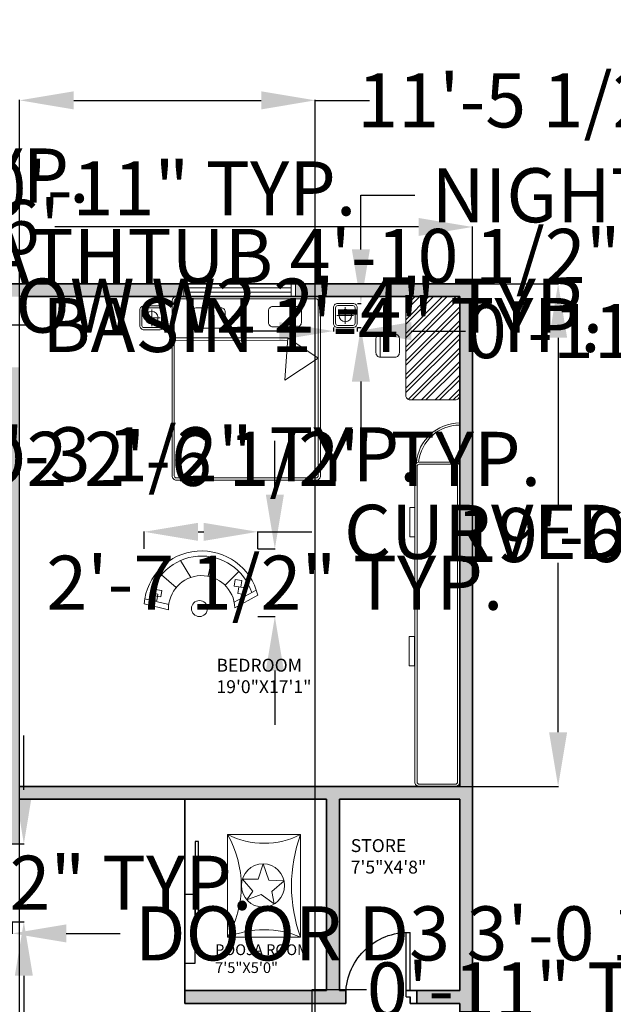
# Model space of a CAD drawing. Units: inches. Extents: x 35 to 5908, y 4 to 3165.
# Tile 5 of 6: x 5270 to 5546, y 2706 to 3165. Entities that reach past the tile are written whole.
import ezdxf

# ---------------------------------------------------------------- set-up
doc = ezdxf.new("R2010")
doc.units = ezdxf.units.IN
doc.header["$MEASUREMENT"] = 0
for name, color, linetype, lineweight in [('A-ANNO-DIMS', 2, 'Continuous', 18), ('A-DOOR', 4, 'Continuous', 25), ('A-FLOR-CASE', 8, 'Continuous', 18), ('A-FURN', 8, 'Continuous', 18), ('A-FURN-PATT', 9, 'Continuous', 13), ('A-WALL', 7, 'Continuous', 35), ('A-WALL-PATT', 252, 'Continuous', 13)]:
    doc.layers.add(name, color=color, linetype=linetype, lineweight=lineweight)
doc.layers.add('A-AREA-IDEN', color=30, linetype='Continuous', lineweight=18, true_color=0xf8991e)
doc.layers.add('A-GLAZ', color=30, linetype='Continuous', lineweight=18, true_color=0xf8991e)
doc.styles.get("Standard").update_dxf_attribs({"font": 'arial.ttf'})
doc.dimstyles.get("Standard").update_dxf_attribs({"dimtxt": 25.18, "dimasz": 25.18, "dimexe": 0.18, "dimexo": 0.0625, "dimgap": 0.09, "dimtad": 0, "dimtih": 1, "dimtoh": 1, "dimdec": 0, "dimzin": 0, "dimdsep": 46, "dimlunit": 3, "dimtxsty": 'Standard', "dimcen": 0.09, "dimadec": 0, "dimazin": 0, "dimtfac": 1, "dimtdec": 0, "dimtofl": 0, "dimtmove": 0, "dimatfit": 3, "dimfxl": 1, "dimtolj": 1, "dimtzin": 0, "dimarcsym": 0})

# ---------------------------------------------------------------- blocks, each defined once
blk = doc.blocks.new('*D6')
at = {"layer": 'A-ANNO-DIMS', "color": 0, "lineweight": -2, "transparency": 16777216}
for p, q in [((5048.79, 3041.84), (5048.79, 3068.36)), ((5073.97, 3068.18), (5243.35, 3068.18)), ((5455.61, 3068.18), (5286.24, 3068.18)), ((5480.79, 3041.84), (5480.79, 3068.36))]:
    blk.add_line(p, q, dxfattribs=at)
for points in [[(5073.97, 3072.38), (5073.97, 3063.99), (5048.79, 3068.18)], [(5455.61, 3072.38), (5455.61, 3063.99), (5480.79, 3068.18)]]:
    blk.add_solid(points, dxfattribs=at)
at = {"layer": 'Defpoints', "color": 0, "lineweight": -2, "transparency": 16777216}
for p in [(5480.79, 3068.18), (5048.79, 3041.78), (5480.79, 3041.78)]:
    blk.add_point(p, dxfattribs=at)
at = {"layer": 'A-ANNO-DIMS', "color": 0, "transparency": 16777216, "insert": (5264.79, 3068.18), "char_height": 25.18, "attachment_point": 5}
blk.add_mtext("\\A1;36'", dxfattribs=at)
blk = doc.blocks.new('DOOR-30-3-JAMB')
for p, q in [((-2, -27), (-2, 0)), ((0, -30), (0, 0)), ((0, -30), (-2, -30))]:
    blk.add_line(p, q)
blk.add_arc((-1, -29), 29.02, 358.0251, 91.9749)
blk = doc.blocks.new('WINDOW-48')
for p, q in [((0, 0), (0, 6)), ((2, 0), (2, 6)), ((50, 0), (50, 6)), ((52, 0), (52, 6)), ((2, 4), (50, 4)), ((2, 2), (50, 2))]:
    blk.add_line(p, q)
blk = doc.blocks.new('NIGHTSTAND-SQUARE')
for p, q in [((-3.9, 0), (3.83, 0)), ((-0.03, 3.86), (-0.03, -3.96))]:
    blk.add_line(p, q)
for points in [[(-5.56, 3.6, -0.414214), (-3.56, 5.6), (3.56, 5.6, -0.414214), (5.56, 3.6), (5.56, -3.6, -0.414214), (3.56, -5.6), (-3.56, -5.6, -0.414214), (-5.56, -3.6)], [(-4.56, 3.6, -0.414214), (-3.56, 4.6), (3.56, 4.6, -0.414214), (4.56, 3.6), (4.56, -3.6, -0.414214), (3.56, -4.6), (-3.56, -4.6, -0.414214), (-4.56, -3.6)]]:
    blk.add_lwpolyline(points, format="xyb", close=True)
blk.add_circle((0, 0), 2.93)
blk = doc.blocks.new('SEATING-SEMICIRCULAR')
for p, q in [((-8.61, 26.49), (-2.9, 16.18)), ((-6.26, 27.18), (-0.33, 16.47)), ((-10.8, 11.96), (-17.22, 18.38)), ((-15.03, 4.08), (-23.93, 5.87)), ((-14.47, -4.08), (-22.37, -8.78)), ((-9.84, -10.8), (-15.69, -17.74)), ((-4.52, -25.5), (-1.86, -14.3)), ((-2.14, -25.8), (0.56, -14.43))]:
    blk.add_line(p, q)
for points in [[(-12.99, 19.72), (-13.45, 16.67), (-10.4, 16.21), (-9.94, 19.26)], [(-9.61, 21.43), (-10.07, 18.38), (-7.03, 17.91), (-6.56, 20.96)], [(-8.44, -17.54), (-8.91, -20.58), (-5.86, -21.05), (-5.4, -18)], [(-6.7, -19.36), (-7.17, -22.4), (-4.12, -22.87), (-3.66, -19.82)]]:
    blk.add_lwpolyline(points, close=True)
blk.add_circle((0, 0), 3.73)
for radius, start, end in [(26.92, 103.6927, 265.1976), (24.53, 107.9155, 260.4199), (15.45, 91.6667, 271.6667)]:
    blk.add_arc((0.12, 1.02), radius, start, end)
blk = doc.blocks.new('*D20')
at = {"layer": 'A-ANNO-DIMS', "color": 0, "lineweight": -2, "transparency": 16777216}
for p, q in [((5366.93, 2650.28), (5341.75, 2650.28)), ((5392.11, 2652.05), (5392.11, 2650.1)), ((5404.3, 2652.05), (5404.3, 2650.1)), ((5429.48, 2650.28), (5454.66, 2650.28))]:
    blk.add_line(p, q, dxfattribs=at)
for points in [[(5366.93, 2654.48), (5366.93, 2646.08), (5392.11, 2650.28)], [(5429.48, 2654.48), (5429.48, 2646.08), (5404.3, 2650.28)]]:
    blk.add_solid(points, dxfattribs=at)
at = {"layer": 'Defpoints', "color": 0, "lineweight": -2, "transparency": 16777216}
for p in [(5392.11, 2652.11), (5404.3, 2652.11), (5404.3, 2650.28)]:
    blk.add_point(p, dxfattribs=at)
at = {"layer": 'A-ANNO-DIMS', "color": 0, "transparency": 16777216, "insert": (5656.92, 2650.28), "char_height": 25.18, "attachment_point": 5}
blk.add_mtext('\\A1;DINING CHAIR 1\'-0" TYP.', dxfattribs=at)
blk = doc.blocks.new('*D21')
at = {"layer": 'A-ANNO-DIMS', "color": 0, "lineweight": -2, "transparency": 16777216}
for p, q in [((5406.13, 2688.06), (5406.13, 2713.24)), ((5406.13, 2713.24), (5431.31, 2713.24)), ((5404.36, 2662.88), (5406.31, 2662.88)), ((5404.36, 2652.11), (5406.31, 2652.11)), ((5406.13, 2626.93), (5406.13, 2601.75))]:
    blk.add_line(p, q, dxfattribs=at)
for points in [[(5401.93, 2688.06), (5410.32, 2688.06), (5406.13, 2662.88)], [(5401.93, 2626.93), (5410.32, 2626.93), (5406.13, 2652.11)]]:
    blk.add_solid(points, dxfattribs=at)
at = {"layer": 'Defpoints', "color": 0, "lineweight": -2, "transparency": 16777216}
for p in [(5404.3, 2662.88), (5406.13, 2662.88), (5404.3, 2652.11)]:
    blk.add_point(p, dxfattribs=at)
at = {"layer": 'A-ANNO-DIMS', "color": 0, "transparency": 16777216, "insert": (5517.92, 2713.24), "char_height": 25.18, "attachment_point": 5}
blk.add_mtext('\\A1;0\'-11" TYP.', dxfattribs=at)
blk = doc.blocks.new('*D24')
at = {"layer": 'A-ANNO-DIMS', "color": 0, "lineweight": -2, "transparency": 16777216}
for p, q in [((5184.7, 3022.57), (5159.52, 3022.57)), ((5209.88, 3024.93), (5209.88, 3022.39)), ((5226.05, 3024.93), (5226.05, 3022.39)), ((5251.23, 3022.57), (5276.41, 3022.57))]:
    blk.add_line(p, q, dxfattribs=at)
for points in [[(5184.7, 3026.76), (5184.7, 3018.37), (5209.88, 3022.57)], [(5251.23, 3026.76), (5251.23, 3018.37), (5226.05, 3022.57)]]:
    blk.add_solid(points, dxfattribs=at)
at = {"layer": 'Defpoints', "color": 0, "lineweight": -2, "transparency": 16777216}
for p in [(5209.88, 3024.99), (5226.05, 3024.99), (5226.05, 3022.57)]:
    blk.add_point(p, dxfattribs=at)
at = {"layer": 'A-ANNO-DIMS', "color": 0, "transparency": 16777216, "insert": (5410.36, 3022.57), "char_height": 25.18, "attachment_point": 5}
blk.add_mtext('\\A1;BASIN 1\'-4" TYP.', dxfattribs=at)
blk = doc.blocks.new('*D25')
at = {"layer": 'A-ANNO-DIMS', "color": 0, "lineweight": -2, "transparency": 16777216}
for p, q in [((5228.48, 3060.96), (5228.48, 3086.14)), ((5228.48, 3086.14), (5253.66, 3086.14)), ((5226.12, 3035.78), (5228.66, 3035.78)), ((5226.12, 3024.99), (5228.66, 3024.99)), ((5228.48, 2999.81), (5228.48, 2974.63))]:
    blk.add_line(p, q, dxfattribs=at)
for points in [[(5224.28, 3060.96), (5232.68, 3060.96), (5228.48, 3035.78)], [(5224.28, 2999.81), (5232.68, 2999.81), (5228.48, 3024.99)]]:
    blk.add_solid(points, dxfattribs=at)
at = {"layer": 'Defpoints', "color": 0, "lineweight": -2, "transparency": 16777216}
for p in [(5226.05, 3035.78), (5228.48, 3035.78), (5226.05, 3024.99)]:
    blk.add_point(p, dxfattribs=at)
at = {"layer": 'A-ANNO-DIMS', "color": 0, "transparency": 16777216, "insert": (5340.27, 3086.14), "char_height": 25.18, "attachment_point": 5}
blk.add_mtext('\\A1;0\'-11" TYP.', dxfattribs=at)
blk = doc.blocks.new('*D28')
at = {"layer": 'A-ANNO-DIMS', "color": 0, "lineweight": -2, "transparency": 16777216}
for p, q in [((5091.29, 3035.72), (5091.29, 3031.4)), ((5119.29, 3035.72), (5119.29, 3031.4)), ((5066.11, 3031.58), (5040.93, 3031.58)), ((5144.47, 3031.58), (5169.65, 3031.58))]:
    blk.add_line(p, q, dxfattribs=at)
for points in [[(5066.11, 3035.78), (5066.11, 3027.38), (5091.29, 3031.58)], [(5144.47, 3035.78), (5144.47, 3027.38), (5119.29, 3031.58)]]:
    blk.add_solid(points, dxfattribs=at)
at = {"layer": 'Defpoints', "color": 0, "lineweight": -2, "transparency": 16777216}
for p in [(5091.29, 3035.78), (5119.29, 3035.78), (5119.29, 3031.58)]:
    blk.add_point(p, dxfattribs=at)
at = {"layer": 'A-ANNO-DIMS', "color": 0, "transparency": 16777216, "insert": (5360.33, 3031.58), "char_height": 25.18, "attachment_point": 5}
blk.add_mtext('\\A1;WINDOW W2 2\'-4" TYP.', dxfattribs=at)
blk = doc.blocks.new('*D29')
at = {"layer": 'A-ANNO-DIMS', "color": 0, "lineweight": -2, "transparency": 16777216}
for p, q in [((5123.49, 3066.96), (5123.49, 3092.14)), ((5123.49, 3092.14), (5148.67, 3092.14)), ((5119.36, 3041.78), (5123.67, 3041.78)), ((5119.36, 3035.78), (5123.67, 3035.78)), ((5123.49, 3010.6), (5123.49, 2985.42))]:
    blk.add_line(p, q, dxfattribs=at)
for points in [[(5119.3, 3066.96), (5127.69, 3066.96), (5123.49, 3041.78)], [(5119.3, 3010.6), (5127.69, 3010.6), (5123.49, 3035.78)]]:
    blk.add_solid(points, dxfattribs=at)
at = {"layer": 'Defpoints', "color": 0, "lineweight": -2, "transparency": 16777216}
for p in [(5119.29, 3041.78), (5123.49, 3041.78), (5119.29, 3035.78)]:
    blk.add_point(p, dxfattribs=at)
at = {"layer": 'A-ANNO-DIMS', "color": 0, "transparency": 16777216, "insert": (5225.51, 3092.14), "char_height": 25.18, "attachment_point": 5}
blk.add_mtext('\\A1;0\'-6" TYP.', dxfattribs=at)
blk = doc.blocks.new('*D30')
at = {"layer": 'A-ANNO-DIMS', "color": 0, "lineweight": -2, "transparency": 16777216}
for p, q in [((5057.79, 2964.72), (5057.79, 2960.06)), ((5088.07, 2964.72), (5088.07, 2960.06)), ((5032.61, 2960.24), (5007.43, 2960.24)), ((5113.25, 2960.24), (5138.43, 2960.24))]:
    blk.add_line(p, q, dxfattribs=at)
for points in [[(5032.61, 2964.43), (5032.61, 2956.04), (5057.79, 2960.24)], [(5113.25, 2964.43), (5113.25, 2956.04), (5088.07, 2960.24)]]:
    blk.add_solid(points, dxfattribs=at)
at = {"layer": 'Defpoints', "color": 0, "lineweight": -2, "transparency": 16777216}
for p in [(5057.79, 2964.78), (5088.07, 2964.78), (5088.07, 2960.24)]:
    blk.add_point(p, dxfattribs=at)
at = {"layer": 'A-ANNO-DIMS', "color": 0, "transparency": 16777216, "insert": (5329, 2960.24), "char_height": 25.18, "attachment_point": 5}
blk.add_mtext('\\A1;DOOR D2 2\'-6 1/2" TYP.', dxfattribs=at)
blk = doc.blocks.new('*D32')
at = {"layer": 'A-ANNO-DIMS', "color": 0, "lineweight": -2, "transparency": 16777216}
for p, q in [((5230.02, 2744.72), (5230.02, 2739.16)), ((5266.29, 2744.72), (5266.29, 2739.16)), ((5204.84, 2739.34), (5179.66, 2739.34)), ((5291.47, 2739.34), (5316.65, 2739.34))]:
    blk.add_line(p, q, dxfattribs=at)
for points in [[(5204.84, 2743.53), (5204.84, 2735.14), (5230.02, 2739.34)], [(5291.47, 2743.53), (5291.47, 2735.14), (5266.29, 2739.34)]]:
    blk.add_solid(points, dxfattribs=at)
at = {"layer": 'Defpoints', "color": 0, "lineweight": -2, "transparency": 16777216}
for p in [(5230.02, 2744.78), (5266.29, 2744.78), (5266.29, 2739.34)]:
    blk.add_point(p, dxfattribs=at)
at = {"layer": 'A-ANNO-DIMS', "color": 0, "transparency": 16777216, "insert": (5507.22, 2739.34), "char_height": 25.18, "attachment_point": 5}
blk.add_mtext('\\A1;DOOR D3 3\'-0 1/2" TYP.', dxfattribs=at)
blk = doc.blocks.new('*D33')
at = {"layer": 'A-ANNO-DIMS', "color": 0, "lineweight": -2, "transparency": 16777216}
for p, q in [((5271.74, 2806.23), (5271.74, 2831.41)), ((5266.36, 2781.05), (5271.92, 2781.05)), ((5266.36, 2744.78), (5271.92, 2744.78)), ((5271.74, 2719.6), (5271.74, 2694.42))]:
    blk.add_line(p, q, dxfattribs=at)
for points in [[(5267.54, 2806.23), (5275.93, 2806.23), (5271.74, 2781.05)], [(5267.54, 2719.6), (5275.93, 2719.6), (5271.74, 2744.78)]]:
    blk.add_solid(points, dxfattribs=at)
at = {"layer": 'Defpoints', "color": 0, "lineweight": -2, "transparency": 16777216}
for p in [(5266.29, 2781.05), (5271.74, 2781.05), (5266.29, 2744.78)]:
    blk.add_point(p, dxfattribs=at)
at = {"layer": 'A-ANNO-DIMS', "color": 0, "transparency": 16777216, "insert": (5271.74, 2762.92), "char_height": 25.18, "attachment_point": 5}
blk.add_mtext('\\A1;3\'-0 1/2" TYP.', dxfattribs=at)
blk = doc.blocks.new('*D34')
at = {"layer": 'A-ANNO-DIMS', "color": 0, "lineweight": -2, "transparency": 16777216}
for p, q in [((5201.71, 3029.52), (5201.71, 3054.7)), ((5201.71, 3054.7), (5226.89, 3054.7)), ((5193.01, 3029.52), (5201.89, 3029.52)), ((5201.71, 2996.29), (5201.71, 3004.34)), ((5193.01, 2971.11), (5201.89, 2971.11))]:
    blk.add_line(p, q, dxfattribs=at)
for points in [[(5197.51, 3004.34), (5205.9, 3004.34), (5201.71, 3029.52)], [(5197.51, 2996.29), (5205.9, 2996.29), (5201.71, 2971.11)]]:
    blk.add_solid(points, dxfattribs=at)
at = {"layer": 'Defpoints', "color": 0, "lineweight": -2, "transparency": 16777216}
for p in [(5192.94, 3029.52), (5201.71, 3029.52), (5192.94, 2971.11)]:
    blk.add_point(p, dxfattribs=at)
at = {"layer": 'A-ANNO-DIMS', "color": 0, "transparency": 16777216, "insert": (5429.25, 3054.7), "char_height": 25.18, "attachment_point": 5}
blk.add_mtext('\\A1;BATHTUB 4\'-10 1/2" TYP.', dxfattribs=at)
blk = doc.blocks.new('*D35')
at = {"layer": 'A-ANNO-DIMS', "color": 0, "lineweight": -2, "transparency": 16777216}
for p, q in [((5165.59, 2971.05), (5165.59, 2962.17)), ((5192.94, 2971.05), (5192.94, 2962.17)), ((5140.41, 2962.35), (5115.23, 2962.35)), ((5218.12, 2962.35), (5243.3, 2962.35))]:
    blk.add_line(p, q, dxfattribs=at)
for points in [[(5140.41, 2966.54), (5140.41, 2958.15), (5165.59, 2962.35)], [(5218.12, 2966.54), (5218.12, 2958.15), (5192.94, 2962.35)]]:
    blk.add_solid(points, dxfattribs=at)
at = {"layer": 'Defpoints', "color": 0, "lineweight": -2, "transparency": 16777216}
for p in [(5165.59, 2971.11), (5192.94, 2971.11), (5192.94, 2962.35)]:
    blk.add_point(p, dxfattribs=at)
at = {"layer": 'A-ANNO-DIMS', "color": 0, "transparency": 16777216, "insert": (5349.69, 2962.35), "char_height": 25.18, "attachment_point": 5}
blk.add_mtext('\\A1;2\'-3 1/2" TYP.', dxfattribs=at)
blk = doc.blocks.new('*D36')
at = {"layer": 'A-ANNO-DIMS', "color": 0, "lineweight": -2, "transparency": 16777216}
for p, q in [((5428.75, 3057.76), (5428.75, 3082.94)), ((5428.75, 3082.94), (5453.93, 3082.94)), ((5427.13, 3032.58), (5428.93, 3032.58)), ((5427.13, 3021.38), (5428.93, 3021.38)), ((5428.75, 2996.2), (5428.75, 2971.02))]:
    blk.add_line(p, q, dxfattribs=at)
for points in [[(5424.55, 3057.76), (5432.94, 3057.76), (5428.75, 3032.58)], [(5424.55, 2996.2), (5432.94, 2996.2), (5428.75, 3021.38)]]:
    blk.add_solid(points, dxfattribs=at)
at = {"layer": 'Defpoints', "color": 0, "lineweight": -2, "transparency": 16777216}
for p in [(5427.07, 3032.58), (5428.75, 3032.58), (5427.07, 3021.38)]:
    blk.add_point(p, dxfattribs=at)
at = {"layer": 'A-ANNO-DIMS', "color": 0, "transparency": 16777216, "insert": (5659.14, 3082.94), "char_height": 25.18, "attachment_point": 5}
blk.add_mtext('\\A1;NIGHTSTAND 0\'-11" TYP.', dxfattribs=at)
blk = doc.blocks.new('*D37')
at = {"layer": 'A-ANNO-DIMS', "color": 0, "lineweight": -2, "transparency": 16777216}
for p, q in [((5415.94, 3021.32), (5415.94, 3019.52)), ((5427.07, 3021.32), (5427.07, 3019.52)), ((5390.76, 3019.7), (5365.58, 3019.7)), ((5452.25, 3019.7), (5477.43, 3019.7))]:
    blk.add_line(p, q, dxfattribs=at)
for points in [[(5390.76, 3023.9), (5390.76, 3015.51), (5415.94, 3019.7)], [(5452.25, 3023.9), (5452.25, 3015.51), (5427.07, 3019.7)]]:
    blk.add_solid(points, dxfattribs=at)
at = {"layer": 'Defpoints', "color": 0, "lineweight": -2, "transparency": 16777216}
for p in [(5415.94, 3021.38), (5427.07, 3021.38), (5427.07, 3019.7)]:
    blk.add_point(p, dxfattribs=at)
at = {"layer": 'A-ANNO-DIMS', "color": 0, "transparency": 16777216, "insert": (5564.04, 3019.7), "char_height": 25.18, "attachment_point": 5}
blk.add_mtext('\\A1;0\'-11" TYP.', dxfattribs=at)
blk = doc.blocks.new('*D40')
at = {"layer": 'A-ANNO-DIMS', "color": 0, "lineweight": -2, "transparency": 16777216}
for p, q in [((5327.75, 2918.38), (5327.75, 2926.45)), ((5352.93, 2926.27), (5355.55, 2926.27)), ((5380.73, 2918.38), (5380.73, 2926.45)), ((5380.73, 2926.27), (5405.91, 2926.27))]:
    blk.add_line(p, q, dxfattribs=at)
for points in [[(5352.93, 2930.46), (5352.93, 2922.07), (5327.75, 2926.27)], [(5355.55, 2930.46), (5355.55, 2922.07), (5380.73, 2926.27)]]:
    blk.add_solid(points, dxfattribs=at)
at = {"layer": 'Defpoints', "color": 0, "lineweight": -2, "transparency": 16777216}
for p in [(5380.73, 2926.27), (5327.75, 2918.32), (5380.73, 2918.32)]:
    blk.add_point(p, dxfattribs=at)
at = {"layer": 'A-ANNO-DIMS', "color": 0, "transparency": 16777216, "insert": (5612.58, 2926.27), "char_height": 25.18, "attachment_point": 5}
blk.add_mtext('\\A1;CURVED SEAT 4\'-5" TYP.', dxfattribs=at)
blk = doc.blocks.new('*D41')
at = {"layer": 'A-ANNO-DIMS', "color": 0, "lineweight": -2, "transparency": 16777216}
for p, q in [((5388.68, 2943.5), (5388.68, 2968.68)), ((5380.8, 2918.32), (5388.86, 2918.32)), ((5380.8, 2886.85), (5388.86, 2886.85)), ((5388.68, 2861.67), (5388.68, 2836.49))]:
    blk.add_line(p, q, dxfattribs=at)
for points in [[(5384.48, 2943.5), (5392.88, 2943.5), (5388.68, 2918.32)], [(5384.48, 2861.67), (5392.88, 2861.67), (5388.68, 2886.85)]]:
    blk.add_solid(points, dxfattribs=at)
at = {"layer": 'Defpoints', "color": 0, "lineweight": -2, "transparency": 16777216}
for p in [(5380.73, 2918.32), (5380.73, 2886.85), (5388.68, 2886.85)]:
    blk.add_point(p, dxfattribs=at)
at = {"layer": 'A-ANNO-DIMS', "color": 0, "transparency": 16777216, "insert": (5388.68, 2902.58), "char_height": 25.18, "attachment_point": 5}
blk.add_mtext('\\A1;2\'-7 1/2" TYP.', dxfattribs=at)
blk = doc.blocks.new('*D47')
at = {"layer": 'A-ANNO-DIMS', "color": 0, "lineweight": -2, "transparency": 16777216}
for p, q in [((5480.86, 3041.78), (5520.82, 3041.78)), ((5520.64, 3016.6), (5520.64, 2937.73)), ((5520.64, 2832.96), (5520.64, 2911.83)), ((5474.86, 2807.78), (5520.82, 2807.78))]:
    blk.add_line(p, q, dxfattribs=at)
for points in [[(5516.45, 3016.6), (5524.84, 3016.6), (5520.64, 3041.78)], [(5516.45, 2832.96), (5524.84, 2832.96), (5520.64, 2807.78)]]:
    blk.add_solid(points, dxfattribs=at)
at = {"layer": 'Defpoints', "color": 0, "lineweight": -2, "transparency": 16777216}
for p in [(5480.79, 3041.78), (5474.79, 2807.78), (5520.64, 2807.78)]:
    blk.add_point(p, dxfattribs=at)
at = {"layer": 'A-ANNO-DIMS', "color": 0, "transparency": 16777216, "insert": (5520.64, 2924.78), "char_height": 25.18, "attachment_point": 5}
blk.add_mtext('\\A1;19\'-6"', dxfattribs=at)
blk = doc.blocks.new('*D50')
at = {"layer": 'A-ANNO-DIMS', "color": 0, "lineweight": -2, "transparency": 16777216}
for p, q in [((5269.79, 2562.84), (5269.79, 3127.3)), ((5294.97, 3127.12), (5382.35, 3127.12)), ((5407.53, 2562.84), (5407.53, 3127.3)), ((5407.53, 3127.12), (5432.71, 3127.12))]:
    blk.add_line(p, q, dxfattribs=at)
for points in [[(5294.97, 3131.32), (5294.97, 3122.92), (5269.79, 3127.12)], [(5382.35, 3131.32), (5382.35, 3122.92), (5407.53, 3127.12)]]:
    blk.add_solid(points, dxfattribs=at)
at = {"layer": 'Defpoints', "color": 0, "lineweight": -2, "transparency": 16777216}
for p in [(5407.53, 3127.12), (5269.79, 2562.78), (5407.53, 2562.78)]:
    blk.add_point(p, dxfattribs=at)
at = {"layer": 'A-ANNO-DIMS', "color": 0, "transparency": 16777216, "insert": (5504.2, 3127.12), "char_height": 25.18, "attachment_point": 5}
blk.add_mtext('\\A1;11\'-5 1/2"', dxfattribs=at)

msp = doc.modelspace()

# ---------------------------------------------------------------- hatches: boundary and pattern name
at = {"layer": 'A-FURN-PATT'}
h = msp.add_hatch(dxfattribs=at)
h.set_pattern_fill('ANSI32', color=256, scale=12)
h.paths.add_polyline_path([(5474.79, 3033.78, 0.414214), (5472.79, 3035.78), (5451.68, 3035.78, 0.414214), (5449.68, 3033.78), (5449.68, 2989.72, 0.414214), (5451.68, 2987.72), (5472.79, 2987.72, 0.414214), (5474.79, 2989.72)])
at = {"layer": 'A-WALL-PATT'}
h = msp.add_hatch(color=256, dxfattribs=at)
h.dxf.hatch_style = 1
h.paths.add_polyline_path([(5198.29, 3041.78), (5119.29, 3041.78), (5119.29, 3035.78), (5155.79, 3035.78), (5155.79, 2967.78), (5087.79, 2967.78), (5087.79, 2966.78, -0.017236), (5087.79, 2964.78), (5087.79, 2961.78), (5262.79, 2961.78), (5262.79, 2967.78), (5236.55, 2967.78), (5236.55, 2967.75), (5218.53, 2967.75), (5161.79, 2967.78), (5161.79, 3035.78), (5198.29, 3035.78)])
h.paths.add_polyline_path([(5091.29, 3041.78), (5048.79, 3041.78), (5048.79, 2877.78), (5054.79, 2877.78), (5054.79, 2899), (5054.79, 2961.78), (5054.79, 2967.78), (5054.79, 3035.78), (5091.29, 3035.78)])
h.paths.add_polyline_path([(5346.29, 3041.78), (5226.29, 3041.78), (5226.29, 3035.78), (5262.79, 3035.78), (5269.79, 3035.78), (5346.29, 3035.78)])
h.paths.add_polyline_path([(5480.79, 3041.78), (5398.29, 3041.78), (5398.29, 3035.78), (5407.91, 3035.78), (5474.79, 3035.78), (5474.79, 2807.78), (5269.79, 2807.78), (5269.79, 3002.78), (5266.29, 3002.78, -0.017236), (5264.29, 3002.78), (5262.79, 3002.78), (5262.79, 2967.78), (5262.79, 2961.78), (5262.79, 2780.78), (5264.29, 2780.78, -0.014283), (5266.29, 2780.78), (5269.79, 2780.78), (5269.79, 2801.78), (5412.79, 2801.78), (5412.79, 2712.78), (5346.79, 2712.78), (5346.79, 2706.78), (5421.79, 2706.78), (5421.79, 2709.78, -0.017236), (5421.79, 2711.78), (5421.79, 2712.78), (5418.79, 2712.78), (5418.79, 2801.78), (5474.79, 2801.78), (5474.79, 2712.78), (5454.79, 2712.78), (5454.79, 2706.78), (5474.79, 2706.78), (5474.79, 2668.42), (5480.79, 2668.42)])
h.paths.add_polyline_path([(5054.79, 2825.78), (5048.79, 2825.78), (5048.79, 2632.28), (5054.79, 2632.28), (5054.79, 2642.69), (5054.79, 2735.78), (5262.79, 2735.78), (5262.79, 2741.78), (5054.79, 2741.78)])
h.paths.add_polyline_path([(5480.79, 2616.42), (5474.79, 2616.42), (5474.79, 2502.2), (5480.79, 2502.2)])
h.paths.add_polyline_path([(5407.53, 2562.78), (5269.79, 2562.78), (5269.79, 2696.78), (5266.29, 2696.78, -0.014283), (5264.29, 2696.78), (5262.79, 2696.78), (5262.79, 2509.78), (5264.29, 2509.78, -0.017236), (5266.29, 2509.78), (5269.79, 2509.78), (5269.79, 2556.78), (5407.53, 2556.78)])
h.paths.add_polyline_path([(5262.79, 2530.78), (5087.79, 2530.78), (5087.79, 2527.78, -0.017236), (5087.79, 2525.78), (5087.79, 2524.78), (5143.79, 2524.78), (5143.79, 2514.78), (5149.79, 2514.78), (5149.79, 2524.78), (5171.79, 2524.78), (5171.79, 2514.78), (5177.79, 2514.78), (5177.79, 2524.78), (5262.79, 2524.78)], flags=17)
h.paths.add_polyline_path([(5262.79, 2395.71), (5262.79, 2321.78), (5480.79, 2321.78), (5480.79, 2450.2), (5474.79, 2450.2), (5474.79, 2381.78), (5425.29, 2381.78), (5425.29, 2375.78), (5474.79, 2375.78), (5474.79, 2327.78), (5269.79, 2327.78), (5269.79, 2375.78), (5312.61, 2375.78), (5312.61, 2381.78), (5269.79, 2381.78), (5269.79, 2395.71)])
h.paths.add_polyline_path([(5171.13, 2321.78), (5171.13, 2327.78), (5054.79, 2327.78), (5054.79, 2470.78), (5157.79, 2470.78), (5262.79, 2470.78), (5262.79, 2461.71), (5269.79, 2461.71), (5269.79, 2476.78), (5262.79, 2476.78), (5177.79, 2476.78), (5177.79, 2486.78), (5171.79, 2486.78), (5171.79, 2476.78), (5149.79, 2476.78), (5149.79, 2486.78), (5143.79, 2486.78), (5143.79, 2476.78), (5054.79, 2476.78), (5054.79, 2580.28), (5048.79, 2580.28), (5048.79, 2321.78)])

# ---------------------------------------------------------------- linework, layer by layer
at = {"layer": 'A-DOOR'}
for points in [[(5351.6, 2746.74), (5353.1, 2746.74), (5353.1, 2782.12), (5351.6, 2782.12)], [(5346.79, 2734.01), (5346.79, 2734.01), (5346.79, 2767.61), (5346.79, 2767.61)], [(5346.79, 2725.56), (5351.6, 2725.56), (5351.6, 2757.46), (5346.79, 2757.46)]]:
    msp.add_lwpolyline(points, close=True, dxfattribs=at)
at = {"layer": 'A-FLOR-CASE'}
for points in [[(5474.79, 2956.72, 0.414214), (5472.79, 2958.72), (5455.93, 2958.72, 0.414214), (5453.93, 2956.72), (5453.93, 2809.78, 0.414214), (5455.93, 2807.78), (5472.79, 2807.78, 0.414214), (5474.79, 2809.78)], [(5473.79, 2956.72, 0.414214), (5472.79, 2957.72), (5455.93, 2957.72, 0.414214), (5454.93, 2956.72), (5454.93, 2809.78, 0.414214), (5455.93, 2808.78), (5472.79, 2808.78, 0.414214), (5473.79, 2809.78)]]:
    msp.add_lwpolyline(points, format="xyb", close=True, dxfattribs=at)
for points in [[(5453.93, 2937.61), (5453.93, 2937.61), (5451.51, 2937.61), (5451.51, 2937.61), (5451.51, 2923.9), (5451.51, 2923.9), (5453.93, 2923.9), (5453.93, 2923.9)], [(5453.72, 2877.53), (5453.72, 2877.53), (5451.3, 2877.53), (5451.3, 2877.53), (5451.3, 2863.83), (5451.3, 2863.83), (5453.72, 2863.83), (5453.72, 2863.83)]]:
    msp.add_lwpolyline(points, close=True, dxfattribs=at)
for radius, end in [(20.24, 175.7422), (19.24, 173.9476)]:
    msp.add_arc((5474.79, 2956.72), radius, 90, end, dxfattribs=at)
at = {"layer": 'A-FURN'}
for p, q in [((5341.84, 3016.65), (5394.67, 3016.65)), ((5393.28, 2996.85), (5394.67, 3016.65)), ((5394.67, 3016.65), (5408.91, 3007.13)), ((5437.8, 3018.26), (5437.8, 3007.6)), ((5341.84, 3015.21), (5394.58, 3015.31)), ((5408.91, 3007.13), (5393.28, 2996.85)), ((5380.84, 2764.56), (5383.17, 2771.71)), ((5383.17, 2771.71), (5385.93, 2764.11)), ((5378.44, 2758.98), (5373.55, 2764.56)), ((5373.55, 2764.56), (5380.84, 2764.56)), ((5385.93, 2764.11), (5393.01, 2763.74)), ((5393.01, 2763.74), (5387.23, 2758.79)), ((5378.44, 2758.98), (5375.66, 2754.99)), ((5375.66, 2754.99), (5382.24, 2757.4)), ((5388.41, 2753.09), (5382.24, 2757.4)), ((5387.23, 2758.79), (5388.41, 2753.09))]:
    msp.add_line(p, q, dxfattribs=at)
for points in [[(5340.84, 3033.78, -0.414214), (5342.84, 3035.78), (5407.91, 3035.78, -0.414214), (5409.91, 3033.78), (5409.91, 2952.35, -0.414214), (5407.91, 2950.35), (5342.84, 2950.35, -0.414214), (5340.84, 2952.35)], [(5341.84, 3033.78, -0.414214), (5342.84, 3034.78), (5407.91, 3034.78, -0.414214), (5408.91, 3033.78), (5408.91, 2952.35, -0.414214), (5407.91, 2951.35), (5342.84, 2951.35, -0.414214), (5341.84, 2952.35)], [(5474.79, 3033.78, 0.414214), (5472.79, 3035.78), (5451.68, 3035.78, 0.414214), (5449.68, 3033.78), (5449.68, 2989.72, 0.414214), (5451.68, 2987.72), (5472.79, 2987.72, 0.414214), (5474.79, 2989.72)], [(5350.2, 3028.59, -0.414214), (5352.2, 3030.59), (5363.51, 3030.59, -0.414214), (5365.51, 3028.59), (5365.51, 3023.06, -0.414214), (5363.51, 3021.06), (5352.2, 3021.06, -0.414214), (5350.2, 3023.06)], [(5385.71, 3029.2, -0.414214), (5387.71, 3031.2), (5399.02, 3031.2, -0.414214), (5401.02, 3029.2), (5401.02, 3023.67, -0.414214), (5399.02, 3021.67), (5387.71, 3021.67, -0.414214), (5385.71, 3023.67)], [(5446.68, 3016.26, 0.414214), (5444.68, 3018.26), (5437.8, 3018.26, 0.414214), (5435.8, 3016.26), (5435.8, 3009.6, 0.414214), (5437.8, 3007.6), (5444.68, 3007.6, 0.414214), (5446.68, 3009.6)]]:
    msp.add_lwpolyline(points, format="xyb", close=True, dxfattribs=at)
msp.add_lwpolyline([(5366.68, 2785.37), (5366.68, 2785.37), (5400.68, 2785.37), (5400.68, 2785.37), (5400.68, 2737.53), (5400.68, 2737.53), (5366.68, 2737.53), (5366.68, 2737.53)], close=True, dxfattribs=at)
msp.add_circle((5383.17, 2761.66), 10.05, dxfattribs=at)
for centre, radius, start, end in [((5383.68, 2818.64), 37.37, 242.9321, 297.0679), ((5324.66, 2761.45), 48.35, 330.3471, 29.6529), ((5465.37, 2761.45), 68.97, 159.7066, 200.2934), ((5383.68, 2698.35), 42.71, 66.5402, 113.4598)]:
    msp.add_arc(centre, radius, start, end, dxfattribs=at)
at = {"layer": 'A-WALL'}
for p, q in [((5048.79, 3041.78), (5480.79, 3041.78)), ((5480.79, 3041.78), (5480.79, 2321.78)), ((5269.79, 3035.78), (5474.79, 3035.78)), ((5474.79, 3035.78), (5474.79, 2807.78)), ((5269.79, 2807.78), (5474.79, 2807.78)), ((5269.79, 2801.78), (5412.79, 2801.78)), ((5346.79, 2712.78), (5346.79, 2801.78)), ((5412.79, 2801.78), (5412.79, 2712.78)), ((5418.79, 2801.78), (5418.79, 2712.78)), ((5418.79, 2801.78), (5474.79, 2801.78)), ((5474.79, 2801.78), (5474.79, 2712.78)), ((5346.79, 2712.78), (5412.79, 2712.78)), ((5346.79, 2712.78), (5346.79, 2706.78)), ((5418.79, 2712.78), (5421.85, 2712.78)), ((5421.79, 2712.78), (5421.79, 2706.78)), ((5449.79, 2712.78), (5474.79, 2712.78)), ((5451.79, 2709.78), (5451.79, 2706.78)), ((5454.79, 2712.78), (5454.79, 2706.78)), ((5346.79, 2706.78), (5421.79, 2706.78)), ((5451.79, 2706.78), (5474.79, 2706.78)), ((5474.79, 2706.78), (5474.79, 2381.78))]:
    msp.add_line(p, q, dxfattribs=at)

# ---------------------------------------------------------------- block references
at = {"layer": 'A-DOOR', "extrusion": (0, 0, -1), "zscale": -1}
msp.add_blockref('DOOR-30-3-JAMB', (-5449.79, 2739.78), dxfattribs=at)
at = {"layer": 'A-FURN'}
for p in [(5331.34, 3025.91), (5421.51, 3026.98)]:
    msp.add_blockref('NIGHTSTAND-SQUARE', p, dxfattribs=at)
at = {"layer": 'A-FURN', "rotation": 270.0000000000218}
msp.add_blockref('SEATING-SEMICIRCULAR', (5353.55, 2890.57), dxfattribs=at)
at = {"layer": 'A-GLAZ'}
msp.add_blockref('WINDOW-48', (5346.3, 3035.78), dxfattribs=at)

# ---------------------------------------------------------------- texts
at = {"layer": 'A-AREA-IDEN', "attachment_point": 1}
for s, insert, char_height in [('BEDROOM\\P19\'0"X17\'1"', (5361.48, 2867.18), 6), ('STORE\\P7\'5"X4\'8"', (5424.03, 2783.21), 6), ('POOJA ROOM\\P7\'5"X5\'0"', (5360.83, 2734.24), 5)]:
    msp.add_mtext_dynamic_manual_height_columns(s, width=69.8687, gutter_width=1, heights=[0], dxfattribs=dict(at, insert=insert, char_height=char_height))

# ---------------------------------------------------------------- dimensions: what is measured, and where the dimension line sits
at = {"layer": 'A-ANNO-DIMS'}
for base, p1, p2, override, picture, middle in [((5407.53, 3127.12), (5269.79, 2562.78), (5407.53, 2562.78), {"dimdec": 1, "dimlfac": 1, "dimrnd": 0, "dimzin": 1, "dimdsep": 46, "dimlunit": 4, "dimfrac": 2}, '*D50', (5504.2, 3127.12)), ((5480.79, 3068.18), (5048.79, 3041.78), (5480.79, 3041.78), {"dimclrd": 0, "dimclre": 0, "dimclrt": 0}, '*D6', (5264.79, 3068.18))]:
    dim = msp.add_linear_dim(base=base, p1=p1, p2=p2, dimstyle='Standard', override=override, dxfattribs=at)
    dim.commit()
    dim.dimension.update_dxf_attribs({"geometry": picture, "text_midpoint": middle})
for base, p1, p2, angle, text, picture, middle in [((5428.75, 3032.58), (5427.07, 3021.38), (5427.07, 3032.58), 90, 'NIGHTSTAND <> TYP.', '*D36', (5659.14, 3082.94)), ((5201.71, 3029.52), (5192.94, 2971.11), (5192.94, 3029.52), 90, 'BATHTUB <> TYP.', '*D34', (5429.25, 3054.7)), ((5123.49, 3041.78), (5119.29, 3035.78), (5119.29, 3041.78), 90, '<> TYP.', '*D29', (5225.51, 3092.14)), ((5228.48, 3035.78), (5226.05, 3024.99), (5226.05, 3035.78), 90, '<> TYP.', '*D25', (5340.27, 3086.14)), ((5380.73, 2926.27), (5327.75, 2918.32), (5380.73, 2918.32), 0, 'CURVED SEAT <> TYP.', '*D40', (5612.58, 2926.27)), ((5388.68, 2886.85), (5380.73, 2918.32), (5380.73, 2886.85), 270, '<> TYP.', '*D41', (5388.68, 2902.58)), ((5271.74, 2781.05), (5266.29, 2744.78), (5266.29, 2781.05), 90, '<> TYP.', '*D33', (5271.74, 2762.92)), ((5406.13, 2662.88), (5404.3, 2652.11), (5404.3, 2662.88), 90, '<> TYP.', '*D21', (5517.92, 2713.24))]:
    dim = msp.add_linear_dim(base=base, p1=p1, p2=p2, angle=angle, text=text, dimstyle='Standard', override={"dimdec": 1, "dimlfac": 1, "dimrnd": 0, "dimzin": 1, "dimdsep": 46, "dimlunit": 4, "dimfrac": 2}, dxfattribs=at)
    dim.commit()
    dim.dimension.update_dxf_attribs({"geometry": picture, "text_midpoint": middle})
for base, p1, p2, text, picture, middle in [((5119.29, 3031.58), (5091.29, 3035.78), (5119.29, 3035.78), 'WINDOW W2 <> TYP.', '*D28', (5360.33, 3031.58)), ((5226.05, 3022.57), (5209.88, 3024.99), (5226.05, 3024.99), 'BASIN <> TYP.', '*D24', (5410.36, 3022.57)), ((5088.07, 2960.24), (5057.79, 2964.78), (5088.07, 2964.78), 'DOOR D2 <> TYP.', '*D30', (5329, 2960.24)), ((5427.07, 3019.7), (5415.94, 3021.38), (5427.07, 3021.38), '<> TYP.', '*D37', (5564.04, 3019.7)), ((5192.9443, 2962.3472), (5165.5853, 2971.109), (5192.9443, 2971.109), '<> TYP.', '*D35', (5349.6879, 2962.3472)), ((5266.29, 2739.34), (5230.02, 2744.78), (5266.29, 2744.78), 'DOOR D3 <> TYP.', '*D32', (5507.22, 2739.34)), ((5404.3, 2650.28), (5392.11, 2652.11), (5404.3, 2652.11), 'DINING CHAIR <> TYP.', '*D20', (5656.92, 2650.28))]:
    dim = msp.add_linear_dim(base=base, p1=p1, p2=p2, text=text, dimstyle='Standard', override={"dimdec": 1, "dimlfac": 1, "dimrnd": 0, "dimzin": 1, "dimdsep": 46, "dimlunit": 4, "dimfrac": 2}, dxfattribs=at)
    dim.commit()
    dim.dimension.update_dxf_attribs({"geometry": picture, "text_midpoint": middle})
dim = msp.add_linear_dim(base=(5520.64, 2807.78), p1=(5480.79, 3041.78), p2=(5474.79, 2807.78), angle=90, dimstyle='Standard', override={"dimdec": 1, "dimlfac": 1, "dimrnd": 0, "dimzin": 1, "dimdsep": 46, "dimlunit": 4, "dimfrac": 2}, dxfattribs=at)
dim.commit()
dim.dimension.update_dxf_attribs({"geometry": '*D47', "text_midpoint": (5520.64, 2924.78)})

doc.saveas('drawing.dxf')
